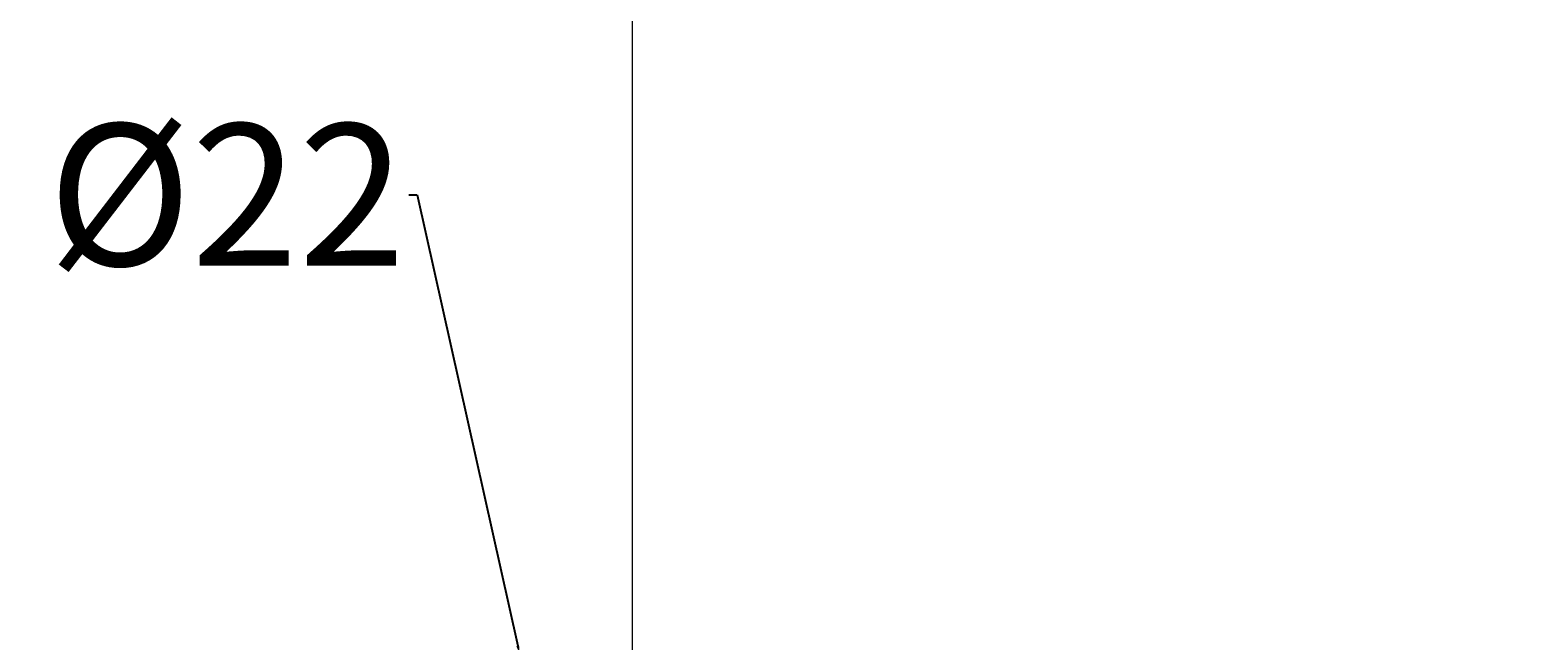
# Model space of a CAD drawing. Units: millimetres. Extents: x -53 to 92, y -147 to 37.
# Tile 8 of 16: x 6 to 38, y -43 to -30. Entities that reach past the tile are written whole.
import ezdxf

# ---------------------------------------------------------------- set-up
doc = ezdxf.new("R2010")
doc.units = ezdxf.units.MM
doc.header["$MEASUREMENT"] = 0
doc.linetypes.add('CENTER', pattern=[50.8, 31.75, -6.35, 6.35, -6.35])
for name, color, linetype, lineweight in [('M-CNTR', 4, 'CENTER', 18), ('M-DIMS', 2, 'Continuous', 25), ('M-OUTL', 7, 'Continuous', 50)]:
    doc.layers.add(name, color=color, linetype=linetype, lineweight=lineweight)
doc.styles.get("Standard").update_dxf_attribs({"font": 'arial.ttf'})
doc.dimstyles.get("Standard").update_dxf_attribs({"dimtxt": 0.18, "dimasz": 0.18, "dimexe": 0.18, "dimexo": 0.0625, "dimgap": 0.09, "dimtad": 0, "dimtih": 1, "dimtoh": 1, "dimdec": 4, "dimzin": 0, "dimdsep": 46, "dimtxsty": 'Standard', "dimcen": 0.09, "dimadec": 0, "dimazin": 0, "dimtfac": 1, "dimtdec": 4, "dimtofl": 0, "dimtmove": 0, "dimatfit": 3, "dimfxl": 1, "dimtolj": 1, "dimtzin": 0, "dimarcsym": 0})

# ---------------------------------------------------------------- blocks, each defined once
blk = doc.blocks.new('*D7')
at = {"layer": 'Defpoints', "color": 0, "transparency": 16777216}
for p in [(9.445, -3.88), (-44.321, -53.98), (18.956, -53.98)]:
    blk.add_point(p, dxfattribs=at)
at = {"layer": 'M-DIMS', "color": 0, "lineweight": -2, "transparency": 16777216}
for p, q in [((9.382, -3.88), (-44.501, -3.88)), ((-44.321, -4.06), (-44.321, -27.308)), ((-44.321, -53.8), (-44.321, -30.552)), ((18.894, -53.98), (-44.501, -53.98))]:
    blk.add_line(p, q, dxfattribs=at)
at = {"layer": 'M-DIMS', "color": 0, "transparency": 16777216}
for points in [[(-44.351, -4.06), (-44.291, -4.06), (-44.321, -3.88)], [(-44.351, -53.8), (-44.291, -53.8), (-44.321, -53.98)]]:
    blk.add_solid(points, dxfattribs=at)
at = {"layer": 'M-DIMS', "color": 0, "transparency": 16777216, "insert": (-44.321, -28.93), "char_height": 0.18, "attachment_point": 5}
blk.add_mtext('\\A1;{\\H16.66667x;50}', dxfattribs=at)
blk = doc.blocks.new('*D10')
at = {"layer": 'Defpoints', "color": 0, "transparency": 16777216}
for p in [(64.593, -18.184), (-26.68, -89.776)]:
    blk.add_point(p, dxfattribs=at)
at = {"layer": 'M-DIMS', "color": 0, "lineweight": -2, "transparency": 16777216}
for p, q in [((77.384, -8.151), (64.734, -18.073)), ((77.564, -8.151), (77.384, -8.151)), ((18.866, -53.98), (19.046, -53.98)), ((18.956, -54.07), (18.956, -53.89))]:
    blk.add_line(p, q, dxfattribs=at)
at = {"layer": 'M-DIMS', "color": 0, "transparency": 16777216}
blk.add_solid([(64.716, -18.05), (64.753, -18.097), (64.593, -18.184)], dxfattribs=at)
at = {"layer": 'M-DIMS', "color": 0, "transparency": 16777216, "insert": (82.599, -8.151), "char_height": 0.18, "attachment_point": 5}
blk.add_mtext('\\A1;{\\H16.66667x;%%C116}', dxfattribs=at)
blk = doc.blocks.new('*D13')
at = {"layer": 'Defpoints', "color": 0, "transparency": 16777216}
for p in [(16.562, -43.244), (21.351, -64.716)]:
    blk.add_point(p, dxfattribs=at)
at = {"layer": 'M-DIMS', "color": 0, "lineweight": -2, "transparency": 16777216}
for p, q in [((14.214, -33.523), (14.394, -33.523)), ((14.394, -33.523), (16.523, -43.068)), ((18.866, -53.98), (19.046, -53.98)), ((18.956, -54.07), (18.956, -53.89))]:
    blk.add_line(p, q, dxfattribs=at)
at = {"layer": 'M-DIMS', "color": 0, "transparency": 16777216}
blk.add_solid([(16.552, -43.062), (16.494, -43.075), (16.562, -43.244)], dxfattribs=at)
at = {"layer": 'M-DIMS', "color": 0, "transparency": 16777216, "insert": (10.359, -33.523), "char_height": 0.18, "attachment_point": 5}
blk.add_mtext('\\A1;{\\H16.66667x;%%C22}', dxfattribs=at)
blk = doc.blocks.new('*D17')
at = {"layer": 'Defpoints', "color": 0, "transparency": 16777216}
for p in [(-46.81, 25.909), (28.564, 25.909), (18.165, -111.975)]:
    blk.add_point(p, dxfattribs=at)
at = {"layer": 'M-DIMS', "color": 0, "lineweight": -2, "transparency": 16777216}
for p, q in [((28.502, 25.909), (-46.99, 25.909)), ((-46.81, 25.729), (-46.81, -42.851)), ((-46.81, -111.795), (-46.81, -43.215)), ((18.102, -111.975), (-46.99, -111.975))]:
    blk.add_line(p, q, dxfattribs=at)
at = {"layer": 'M-DIMS', "color": 0, "transparency": 16777216}
for points in [[(-46.84, 25.729), (-46.78, 25.729), (-46.81, 25.909)], [(-46.84, -111.795), (-46.78, -111.795), (-46.81, -111.975)]]:
    blk.add_solid(points, dxfattribs=at)
at = {"layer": 'M-DIMS', "color": 0, "transparency": 16777216, "insert": (-46.81, -43.033), "char_height": 0.18, "attachment_point": 5}
blk.add_mtext('\\A1;137.88', dxfattribs=at)
blk = doc.blocks.new('*D18')
at = {"layer": 'Defpoints', "color": 0, "transparency": 16777216}
for p in [(19.753, 4.014), (18.16, -111.975)]:
    blk.add_point(p, dxfattribs=at)
at = {"layer": 'M-DIMS', "color": 0, "lineweight": -2, "transparency": 16777216}
for p, q in [((18.866, -53.98), (19.046, -53.98)), ((18.956, -54.07), (18.956, -53.89)), ((17.682, -146.771), (18.158, -112.155)), ((17.502, -146.771), (17.682, -146.771))]:
    blk.add_line(p, q, dxfattribs=at)
at = {"layer": 'M-DIMS', "color": 0, "transparency": 16777216}
blk.add_solid([(18.128, -112.154), (18.188, -112.155), (18.16, -111.975)], dxfattribs=at)
at = {"layer": 'M-DIMS', "color": 0, "transparency": 16777216, "insert": (17.115, -146.771), "char_height": 0.18, "attachment_point": 5}
blk.add_mtext('\\A1;∅116', dxfattribs=at)

msp = doc.modelspace()

# ---------------------------------------------------------------- linework, layer by layer
at = {"layer": 'M-CNTR'}
msp.add_line((18.95638, -54.07007), (18.95638, -15.58399), dxfattribs=at)
at = {"layer": 'M-OUTL'}
msp.add_arc((18.95638, -53.98007), 58, 108.3895553, 70.0459142, dxfattribs=at)

# ---------------------------------------------------------------- dimensions: what is measured, and where the dimension line sits
at = {"layer": 'M-DIMS'}
dim = msp.add_linear_dim(base=(-46.8103, 25.90924), p1=(18.16452, -111.97467), p2=(28.56407, 25.90924), angle=90, dimstyle='Standard', override={"dimdec": 2, "dimlfac": 1, "dimrnd": 0, "dimzin": 0, "dimdsep": 46, "dimlunit": 2}, dxfattribs=at)
dim.commit()
dim.dimension.update_dxf_attribs({"geometry": '*D17', "text_midpoint": (-46.8103, -43.03271)})
dim = msp.add_diameter_dim_2p(p1=(19.75275, 4.01446), p2=(18.16001, -111.9746), dimstyle='Standard', override={"dimdec": 0, "dimlfac": 1, "dimrnd": 0, "dimzin": 0, "dimdsep": 46, "dimlunit": 2}, dxfattribs=at)
dim.commit()
dim.dimension.update_dxf_attribs({"geometry": '*D18', "text_midpoint": (17.11548, -146.77132), "dimtype": 163})
dim = msp.add_linear_dim(base=(-44.32095, -53.98007), p1=(9.44461, -3.87977), p2=(18.95638, -53.98007), angle=90, text='{\\H16.66667x;50}', dimstyle='Standard', override={"dimclrd": 0, "dimclre": 0, "dimclrt": 0}, dxfattribs=at)
dim.commit()
dim.dimension.update_dxf_attribs({"geometry": '*D7', "text_midpoint": (-44.32095, -28.92992)})
for p1, p2, text, picture, middle in [((-26.67986, -89.77579), (64.59262, -18.18435), '{\\H16.66667x;%%C116}', '*D10', (82.59889, -8.15132)), ((21.35078, -64.71631), (16.56198, -43.24383), '{\\H16.66667x;%%C22}', '*D13', (10.35867, -33.52288))]:
    dim = msp.add_diameter_dim_2p(p1=p1, p2=p2, text=text, dimstyle='Standard', override={"dimclrd": 0, "dimclre": 0, "dimclrt": 0}, dxfattribs=at)
    dim.commit()
    dim.dimension.update_dxf_attribs({"geometry": picture, "text_midpoint": middle, "dimtype": 163})

doc.saveas('drawing.dxf')
